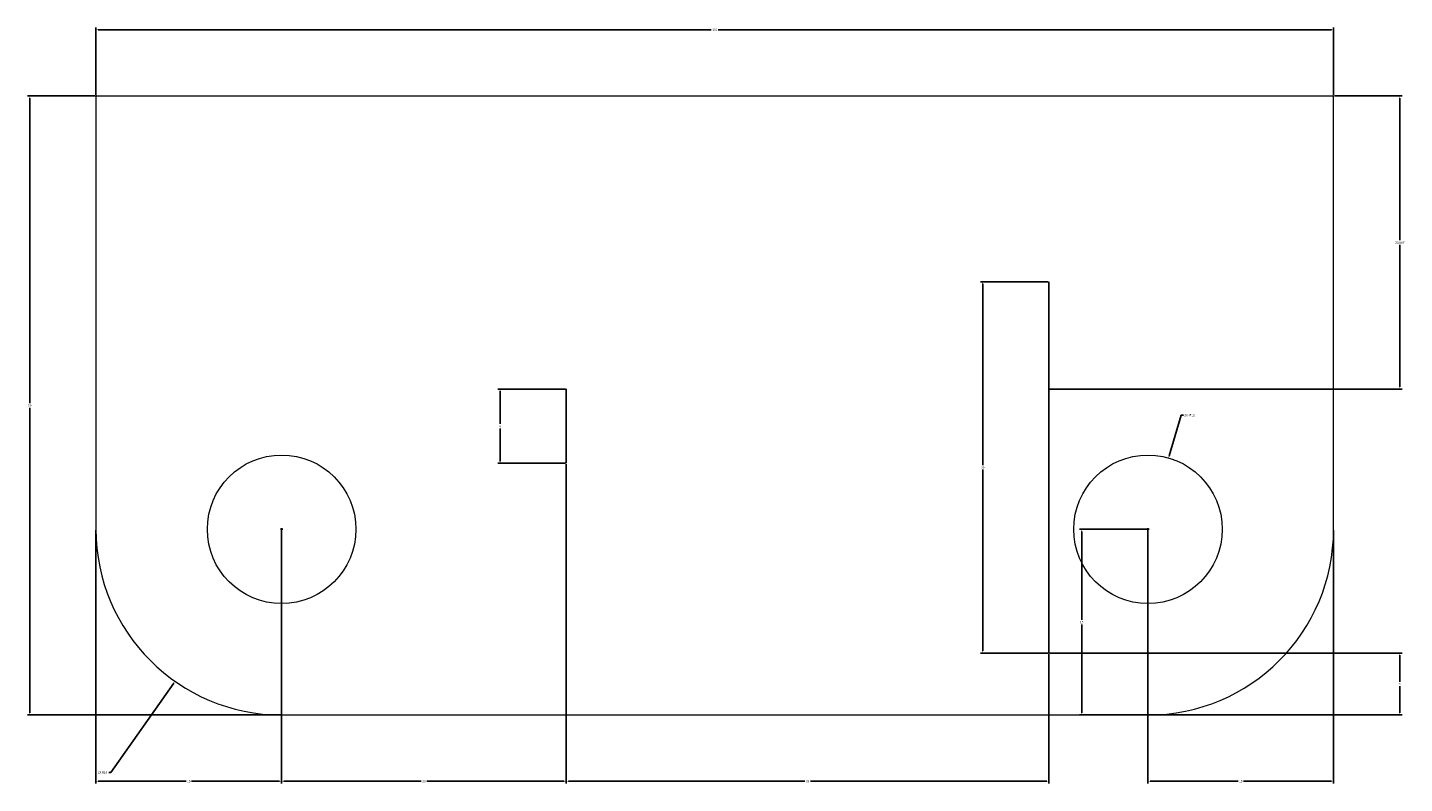
# Model space of a CAD drawing. Units: millimetres. Extents: x -5 to 2707, y 665 to 1247.
# Tile 3 of 3: x 2481 to 2592, y 1186 to 1247. Entities that reach past the tile are written whole.
import ezdxf

# ---------------------------------------------------------------- set-up
doc = ezdxf.new("R2010")
doc.units = ezdxf.units.MM
doc.layers.add('M-CONS', color=7, linetype='Continuous', lineweight=18)
doc.layers.add('M-DIMS', color=2, linetype='Continuous', lineweight=18)
doc.styles.get("Standard").update_dxf_attribs({"font": 'arial.ttf'})
doc.dimstyles.get("Standard").update_dxf_attribs({"dimtxt": 0.18, "dimasz": 0.18, "dimexe": 0.18, "dimexo": 0.0625, "dimgap": 0.09, "dimtad": 0, "dimtih": 1, "dimtoh": 1, "dimdec": 4, "dimzin": 0, "dimdsep": 46, "dimtxsty": 'Standard', "dimcen": 0.09, "dimadec": 0, "dimazin": 0, "dimtfac": 1, "dimtdec": 4, "dimtofl": 0, "dimtmove": 0, "dimatfit": 3, "dimfxl": 1, "dimtolj": 1, "dimtzin": 0, "dimarcsym": 0})

# ---------------------------------------------------------------- blocks, each defined once
blk = doc.blocks.new('*D1')
at = {"layer": 'Defpoints', "color": 0, "transparency": 16777216}
for p in [(2586.43, 1246.7), (2486.43, 1241.35), (2586.43, 1241.35)]:
    blk.add_point(p, dxfattribs=at)
at = {"layer": 'M-DIMS', "color": 0, "lineweight": -2, "transparency": 16777216}
for p, q in [((2486.43, 1241.41), (2486.43, 1246.88)), ((2486.61, 1246.7), (2536.15, 1246.7)), ((2586.25, 1246.7), (2536.71, 1246.7)), ((2586.43, 1241.41), (2586.43, 1246.88))]:
    blk.add_line(p, q, dxfattribs=at)
at = {"layer": 'M-DIMS', "color": 0, "transparency": 16777216}
for points in [[(2486.61, 1246.73), (2486.61, 1246.67), (2486.43, 1246.7)], [(2586.25, 1246.73), (2586.25, 1246.67), (2586.43, 1246.7)]]:
    blk.add_solid(points, dxfattribs=at)
at = {"layer": 'M-DIMS', "color": 0, "transparency": 16777216, "insert": (2536.43, 1246.7), "char_height": 0.18, "attachment_point": 5}
blk.add_mtext('\\A1;100', dxfattribs=at)
blk = doc.blocks.new('*D2')
at = {"layer": 'Defpoints', "color": 0, "transparency": 16777216}
for p in [(2486.43, 1241.35), (2481.08, 1191.35), (2501.43, 1191.35)]:
    blk.add_point(p, dxfattribs=at)
at = {"layer": 'M-DIMS', "color": 0, "lineweight": -2, "transparency": 16777216}
for p, q in [((2486.37, 1241.35), (2480.9, 1241.35)), ((2481.08, 1241.17), (2481.08, 1216.53)), ((2481.08, 1191.53), (2481.08, 1216.17)), ((2501.37, 1191.35), (2480.9, 1191.35))]:
    blk.add_line(p, q, dxfattribs=at)
at = {"layer": 'M-DIMS', "color": 0, "transparency": 16777216}
for points in [[(2481.05, 1241.17), (2481.11, 1241.17), (2481.08, 1241.35)], [(2481.05, 1191.53), (2481.11, 1191.53), (2481.08, 1191.35)]]:
    blk.add_solid(points, dxfattribs=at)
at = {"layer": 'M-DIMS', "color": 0, "transparency": 16777216, "insert": (2481.08, 1216.35), "char_height": 0.18, "attachment_point": 5}
blk.add_mtext('\\A1;50', dxfattribs=at)
blk = doc.blocks.new('*D3')
at = {"layer": 'Defpoints', "color": 0, "transparency": 16777216}
for p in [(2519.08, 1217.68), (2524.43, 1217.68), (2524.43, 1211.68)]:
    blk.add_point(p, dxfattribs=at)
at = {"layer": 'M-DIMS', "color": 0, "lineweight": -2, "transparency": 16777216}
for p, q in [((2524.37, 1217.68), (2518.9, 1217.68)), ((2519.08, 1217.5), (2519.08, 1214.86)), ((2519.08, 1211.86), (2519.08, 1214.5)), ((2524.37, 1211.68), (2518.9, 1211.68))]:
    blk.add_line(p, q, dxfattribs=at)
at = {"layer": 'M-DIMS', "color": 0, "transparency": 16777216}
for points in [[(2519.05, 1217.5), (2519.11, 1217.5), (2519.08, 1217.68)], [(2519.05, 1211.86), (2519.11, 1211.86), (2519.08, 1211.68)]]:
    blk.add_solid(points, dxfattribs=at)
at = {"layer": 'M-DIMS', "color": 0, "transparency": 16777216, "insert": (2519.08, 1214.68), "char_height": 0.18, "attachment_point": 5}
blk.add_mtext('\\A1;6', dxfattribs=at)
blk = doc.blocks.new('*D4')
at = {"layer": 'Defpoints', "color": 0, "transparency": 16777216}
for p in [(2524.43, 1211.68), (2501.43, 1206.35), (2524.43, 1186)]:
    blk.add_point(p, dxfattribs=at)
at = {"layer": 'M-DIMS', "color": 0, "lineweight": -2, "transparency": 16777216}
for p, q in [((2524.43, 1211.62), (2524.43, 1185.82)), ((2501.43, 1206.28), (2501.43, 1185.82)), ((2501.61, 1186), (2512.71, 1186)), ((2524.25, 1186), (2513.15, 1186))]:
    blk.add_line(p, q, dxfattribs=at)
at = {"layer": 'M-DIMS', "color": 0, "transparency": 16777216}
for points in [[(2501.61, 1186.03), (2501.61, 1185.97), (2501.43, 1186)], [(2524.25, 1186.03), (2524.25, 1185.97), (2524.43, 1186)]]:
    blk.add_solid(points, dxfattribs=at)
at = {"layer": 'M-DIMS', "color": 0, "transparency": 16777216, "insert": (2512.93, 1186), "char_height": 0.18, "attachment_point": 5}
blk.add_mtext('\\A1;23', dxfattribs=at)
blk = doc.blocks.new('*D5')
at = {"layer": 'Defpoints', "color": 0, "transparency": 16777216}
for p in [(2524.43, 1211.68), (2563.43, 1196.35), (2563.43, 1186)]:
    blk.add_point(p, dxfattribs=at)
at = {"layer": 'M-DIMS', "color": 0, "lineweight": -2, "transparency": 16777216}
for p, q in [((2524.43, 1211.62), (2524.43, 1185.82)), ((2563.43, 1196.28), (2563.43, 1185.82)), ((2524.61, 1186), (2543.71, 1186)), ((2563.25, 1186), (2544.15, 1186))]:
    blk.add_line(p, q, dxfattribs=at)
at = {"layer": 'M-DIMS', "color": 0, "transparency": 16777216}
for points in [[(2524.61, 1186.03), (2524.61, 1185.97), (2524.43, 1186)], [(2563.25, 1186.03), (2563.25, 1185.97), (2563.43, 1186)]]:
    blk.add_solid(points, dxfattribs=at)
at = {"layer": 'M-DIMS', "color": 0, "transparency": 16777216, "insert": (2543.93, 1186), "char_height": 0.18, "attachment_point": 5}
blk.add_mtext('\\A1;39', dxfattribs=at)
blk = doc.blocks.new('*D6')
at = {"layer": 'Defpoints', "color": 0, "transparency": 16777216}
for p in [(2586.43, 1241.35), (2591.78, 1241.35), (2563.43, 1217.68)]:
    blk.add_point(p, dxfattribs=at)
at = {"layer": 'M-DIMS', "color": 0, "lineweight": -2, "transparency": 16777216}
for p, q in [((2586.49, 1241.35), (2591.96, 1241.35)), ((2591.78, 1241.17), (2591.78, 1229.7)), ((2591.78, 1217.86), (2591.78, 1229.33)), ((2563.49, 1217.68), (2591.96, 1217.68))]:
    blk.add_line(p, q, dxfattribs=at)
at = {"layer": 'M-DIMS', "color": 0, "transparency": 16777216}
for points in [[(2591.75, 1241.17), (2591.81, 1241.17), (2591.78, 1241.35)], [(2591.75, 1217.86), (2591.81, 1217.86), (2591.78, 1217.68)]]:
    blk.add_solid(points, dxfattribs=at)
at = {"layer": 'M-DIMS', "color": 0, "transparency": 16777216, "insert": (2591.78, 1229.51), "char_height": 0.18, "attachment_point": 5}
blk.add_mtext('\\A1;23.667', dxfattribs=at)
blk = doc.blocks.new('*D7')
at = {"layer": 'Defpoints', "color": 0, "transparency": 16777216}
for p in [(2558.08, 1226.35), (2563.43, 1226.35), (2563.43, 1196.35)]:
    blk.add_point(p, dxfattribs=at)
at = {"layer": 'M-DIMS', "color": 0, "lineweight": -2, "transparency": 16777216}
for p, q in [((2563.37, 1226.35), (2557.9, 1226.35)), ((2558.08, 1226.17), (2558.08, 1211.53)), ((2558.08, 1196.53), (2558.08, 1211.17)), ((2563.37, 1196.35), (2557.9, 1196.35))]:
    blk.add_line(p, q, dxfattribs=at)
at = {"layer": 'M-DIMS', "color": 0, "transparency": 16777216}
for points in [[(2558.05, 1226.17), (2558.11, 1226.17), (2558.08, 1226.35)], [(2558.05, 1196.53), (2558.11, 1196.53), (2558.08, 1196.35)]]:
    blk.add_solid(points, dxfattribs=at)
at = {"layer": 'M-DIMS', "color": 0, "transparency": 16777216, "insert": (2558.08, 1211.35), "char_height": 0.18, "attachment_point": 5}
blk.add_mtext('\\A1;30', dxfattribs=at)
blk = doc.blocks.new('*D8')
at = {"layer": 'Defpoints', "color": 0, "transparency": 16777216}
for p in [(2563.43, 1196.35), (2571.43, 1191.35), (2591.78, 1191.35)]:
    blk.add_point(p, dxfattribs=at)
at = {"layer": 'M-DIMS', "color": 0, "lineweight": -2, "transparency": 16777216}
for p, q in [((2563.49, 1196.35), (2591.96, 1196.35)), ((2591.78, 1196.17), (2591.78, 1194.03)), ((2591.78, 1191.53), (2591.78, 1193.67)), ((2571.49, 1191.35), (2591.96, 1191.35))]:
    blk.add_line(p, q, dxfattribs=at)
at = {"layer": 'M-DIMS', "color": 0, "transparency": 16777216}
for points in [[(2591.75, 1196.17), (2591.81, 1196.17), (2591.78, 1196.35)], [(2591.75, 1191.53), (2591.81, 1191.53), (2591.78, 1191.35)]]:
    blk.add_solid(points, dxfattribs=at)
at = {"layer": 'M-DIMS', "color": 0, "transparency": 16777216, "insert": (2591.78, 1193.85), "char_height": 0.18, "attachment_point": 5}
blk.add_mtext('\\A1;5', dxfattribs=at)
blk = doc.blocks.new('*D9')
at = {"layer": 'Defpoints', "color": 0, "transparency": 16777216}
for p in [(2571.43, 1206.35), (2586.43, 1206.35), (2586.43, 1186)]:
    blk.add_point(p, dxfattribs=at)
at = {"layer": 'M-DIMS', "color": 0, "lineweight": -2, "transparency": 16777216}
for p, q in [((2571.43, 1206.28), (2571.43, 1185.82)), ((2586.43, 1206.28), (2586.43, 1185.82)), ((2571.61, 1186), (2578.72, 1186)), ((2586.25, 1186), (2579.14, 1186))]:
    blk.add_line(p, q, dxfattribs=at)
at = {"layer": 'M-DIMS', "color": 0, "transparency": 16777216}
for points in [[(2571.61, 1186.03), (2571.61, 1185.97), (2571.43, 1186)], [(2586.25, 1186.03), (2586.25, 1185.97), (2586.43, 1186)]]:
    blk.add_solid(points, dxfattribs=at)
at = {"layer": 'M-DIMS', "color": 0, "transparency": 16777216, "insert": (2578.93, 1186), "char_height": 0.18, "attachment_point": 5}
blk.add_mtext('\\A1;15', dxfattribs=at)
blk = doc.blocks.new('*D10')
at = {"layer": 'Defpoints', "color": 0, "transparency": 16777216}
for p in [(2486.43, 1206.35), (2501.43, 1206.35), (2501.43, 1186)]:
    blk.add_point(p, dxfattribs=at)
at = {"layer": 'M-DIMS', "color": 0, "lineweight": -2, "transparency": 16777216}
for p, q in [((2486.43, 1206.28), (2486.43, 1185.82)), ((2501.43, 1206.28), (2501.43, 1185.82)), ((2486.61, 1186), (2493.72, 1186)), ((2501.25, 1186), (2494.14, 1186))]:
    blk.add_line(p, q, dxfattribs=at)
at = {"layer": 'M-DIMS', "color": 0, "transparency": 16777216}
for points in [[(2486.61, 1186.03), (2486.61, 1185.97), (2486.43, 1186)], [(2501.25, 1186.03), (2501.25, 1185.97), (2501.43, 1186)]]:
    blk.add_solid(points, dxfattribs=at)
at = {"layer": 'M-DIMS', "color": 0, "transparency": 16777216, "insert": (2493.93, 1186), "char_height": 0.18, "attachment_point": 5}
blk.add_mtext('\\A1;15', dxfattribs=at)
blk = doc.blocks.new('*D11')
at = {"layer": 'Defpoints', "color": 0, "transparency": 16777216}
for p in [(2566.08, 1206.35), (2571.43, 1206.35), (2571.43, 1191.35)]:
    blk.add_point(p, dxfattribs=at)
at = {"layer": 'M-DIMS', "color": 0, "lineweight": -2, "transparency": 16777216}
for p, q in [((2571.37, 1206.35), (2565.9, 1206.35)), ((2566.08, 1206.17), (2566.08, 1199.03)), ((2566.08, 1191.53), (2566.08, 1198.67)), ((2571.37, 1191.35), (2565.9, 1191.35))]:
    blk.add_line(p, q, dxfattribs=at)
at = {"layer": 'M-DIMS', "color": 0, "transparency": 16777216}
for points in [[(2566.05, 1206.17), (2566.11, 1206.17), (2566.08, 1206.35)], [(2566.05, 1191.53), (2566.11, 1191.53), (2566.08, 1191.35)]]:
    blk.add_solid(points, dxfattribs=at)
at = {"layer": 'M-DIMS', "color": 0, "transparency": 16777216, "insert": (2566.08, 1198.85), "char_height": 0.18, "attachment_point": 5}
blk.add_mtext('\\A1;15', dxfattribs=at)
blk = doc.blocks.new('*D16')
at = {"layer": 'Defpoints', "color": 0, "transparency": 16777216}
for p in [(2573.1, 1212.11), (2569.76, 1200.59)]:
    blk.add_point(p, dxfattribs=at)
at = {"layer": 'M-DIMS', "color": 0, "lineweight": -2, "transparency": 16777216}
for p, q in [((2574.11, 1215.57), (2573.15, 1212.28)), ((2574.29, 1215.57), (2574.11, 1215.57)), ((2571.34, 1206.35), (2571.52, 1206.35)), ((2571.43, 1206.26), (2571.43, 1206.44))]:
    blk.add_line(p, q, dxfattribs=at)
at = {"layer": 'M-DIMS', "color": 0, "transparency": 16777216}
blk.add_solid([(2573.12, 1212.29), (2573.18, 1212.27), (2573.1, 1212.11)], dxfattribs=at)
at = {"layer": 'M-DIMS', "color": 0, "transparency": 16777216, "insert": (2574.79, 1215.57), "char_height": 0.18, "attachment_point": 5}
blk.add_mtext('\\A1;2X ∅12', dxfattribs=at)
blk = doc.blocks.new('*D17')
at = {"layer": 'Defpoints', "color": 0, "transparency": 16777216}
for p in [(2501.43, 1206.35), (2492.81, 1194.07)]:
    blk.add_point(p, dxfattribs=at)
at = {"layer": 'M-DIMS', "color": 0, "lineweight": -2, "transparency": 16777216}
for p, q in [((2501.34, 1206.35), (2501.52, 1206.35)), ((2501.43, 1206.26), (2501.43, 1206.44)), ((2487.64, 1186.71), (2492.71, 1193.93)), ((2487.46, 1186.71), (2487.64, 1186.71))]:
    blk.add_line(p, q, dxfattribs=at)
at = {"layer": 'M-DIMS', "color": 0, "transparency": 16777216}
blk.add_solid([(2492.68, 1193.94), (2492.73, 1193.91), (2492.81, 1194.07)], dxfattribs=at)
at = {"layer": 'M-DIMS', "color": 0, "transparency": 16777216, "insert": (2486.96, 1186.71), "char_height": 0.18, "attachment_point": 5}
blk.add_mtext('\\A1;2X R15', dxfattribs=at)

msp = doc.modelspace()

# ---------------------------------------------------------------- linework, layer by layer
at = {"layer": 'M-CONS'}
msp.add_lwpolyline([(2586.4304, 1241.3473), (2486.4304, 1241.3473), (2486.4304, 1206.3473, 0.41421356), (2501.4304, 1191.3473), (2571.4304, 1191.3473, 0.41421356), (2586.4304, 1206.3473)], format="xyb", close=True, dxfattribs=at)
msp.add_polyline3d([(2563.4304, 1226.3473, 30), (2563.4304, 1226.3473, 50), (2563.4304, 1211.3473, 50), (2563.4304, 1196.3473, 30)], close=True, dxfattribs=at)
at = {"layer": 'M-CONS', "extrusion": (1, 0, 0)}
for centre in [(1214.6807, 38.8889, 2524.4304), (1214.6807, 38.8889, 2563.4304)]:
    msp.add_circle(centre, 3, dxfattribs=at)
at = {"layer": 'M-CONS'}
for centre in [(2501.4304, 1206.3473), (2571.4304, 1206.3473)]:
    msp.add_circle(centre, 6, dxfattribs=at)

# ---------------------------------------------------------------- dimensions: what is measured, and where the dimension line sits
at = {"layer": 'M-DIMS'}
for base, p1, p2, picture, middle in [((2586.4304, 1246.6973), (2486.4304, 1241.3473), (2586.4304, 1241.3473), '*D1', (2536.4304, 1246.6973)), ((2524.4304, 1185.9973), (2501.4304, 1206.3473), (2524.4304, 1211.6807), '*D4', (2512.9304, 1185.9973)), ((2563.4304, 1185.9973), (2524.4304, 1211.6807), (2563.4304, 1196.3473), '*D5', (2543.9304, 1185.9973)), ((2501.4304, 1185.9973), (2486.4304, 1206.3473), (2501.4304, 1206.3473), '*D10', (2493.9304, 1185.9973)), ((2586.4304, 1185.9973), (2571.4304, 1206.3473), (2586.4304, 1206.3473), '*D9', (2578.9304, 1185.9973))]:
    dim = msp.add_linear_dim(base=base, p1=p1, p2=p2, dimstyle='Standard', override={"dimdec": 0, "dimlfac": 1, "dimrnd": 0, "dimzin": 0, "dimdsep": 46, "dimlunit": 2}, dxfattribs=at)
    dim.commit()
    dim.dimension.update_dxf_attribs({"geometry": picture, "text_midpoint": middle})
for base, p1, p2, override, picture, middle in [((2481.0804, 1191.3473), (2486.4304, 1241.3473), (2501.4304, 1191.3473), {"dimdec": 0, "dimlfac": 1, "dimrnd": 0, "dimzin": 0, "dimdsep": 46, "dimlunit": 2}, '*D2', (2481.0804, 1216.3473)), ((2591.7804, 1241.3473), (2563.4304, 1217.6807), (2586.4304, 1241.3473), {"dimdec": 3, "dimlfac": 1, "dimrnd": 0, "dimzin": 0, "dimdsep": 46, "dimlunit": 2}, '*D6', (2591.7804, 1229.514)), ((2558.0804, 1226.3473), (2563.4304, 1196.3473), (2563.4304, 1226.3473), {"dimdec": 0, "dimlfac": 1, "dimrnd": 0, "dimzin": 0, "dimdsep": 46, "dimlunit": 2}, '*D7', (2558.0804, 1211.3473)), ((2519.0804, 1217.6807), (2524.4304, 1211.6807), (2524.4304, 1217.6807), {"dimdec": 0, "dimlfac": 1, "dimrnd": 0, "dimzin": 0, "dimdsep": 46, "dimlunit": 2}, '*D3', (2519.0804, 1214.6807)), ((2566.0804, 1206.3473), (2571.4304, 1191.3473), (2571.4304, 1206.3473), {"dimdec": 0, "dimlfac": 1, "dimrnd": 0, "dimzin": 0, "dimdsep": 46, "dimlunit": 2}, '*D11', (2566.0804, 1198.8473)), ((2591.7804, 1191.3473), (2563.4304, 1196.3473), (2571.4304, 1191.3473), {"dimdec": 0, "dimlfac": 1, "dimrnd": 0, "dimzin": 0, "dimdsep": 46, "dimlunit": 2}, '*D8', (2591.7804, 1193.8473))]:
    dim = msp.add_linear_dim(base=base, p1=p1, p2=p2, angle=90, dimstyle='Standard', override=override, dxfattribs=at)
    dim.commit()
    dim.dimension.update_dxf_attribs({"geometry": picture, "text_midpoint": middle})
dim = msp.add_diameter_dim_2p(p1=(2569.7581, 1200.5851), p2=(2573.1028, 1212.1096), text='2X <>', dimstyle='Standard', override={"dimdec": 0, "dimlfac": 1, "dimrnd": 0, "dimzin": 0, "dimdsep": 46, "dimlunit": 2}, dxfattribs=at)
dim.commit()
dim.dimension.update_dxf_attribs({"geometry": '*D16', "text_midpoint": (2574.7922, 1215.5669), "dimtype": 163})
dim = msp.add_radius_dim(center=(2501.4304, 1206.3473), mpoint=(2492.8089, 1194.0726), text='2X <>', dimstyle='Standard', override={"dimdec": 0, "dimlfac": 1, "dimrnd": 0, "dimzin": 0, "dimdsep": 46, "dimlunit": 2}, dxfattribs=at)
dim.commit()
dim.dimension.update_dxf_attribs({"geometry": '*D17', "text_midpoint": (2486.9553, 1186.7078), "dimtype": 164})

doc.saveas('drawing.dxf')
